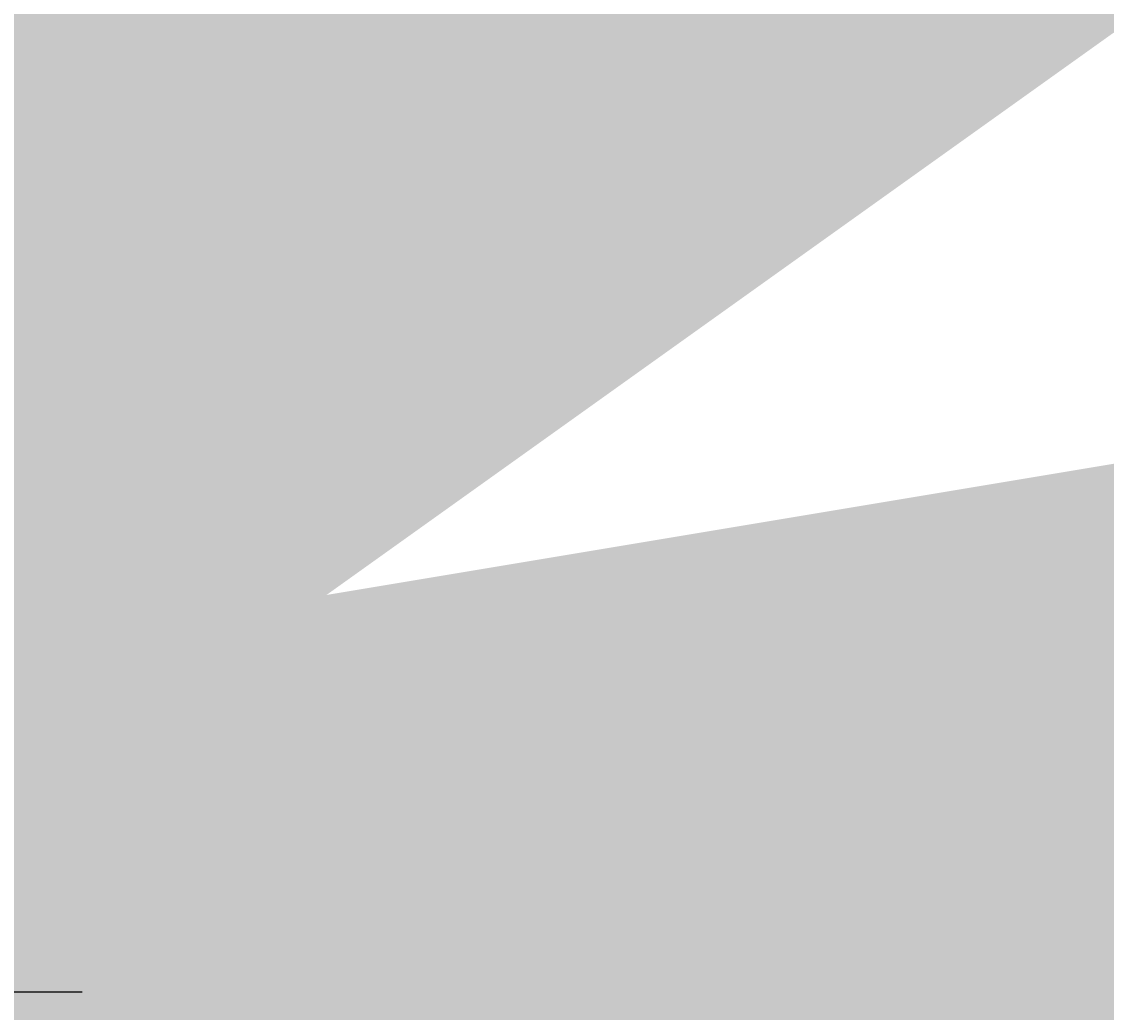
# Model space of a CAD drawing. Units: millimetres. Extents: x -22994 to 29398, y -19990 to 20176.
# Tile 126 of 135: x 296 to 480, y 173 to 341. Entities that reach past the tile are written whole.
import ezdxf

# ---------------------------------------------------------------- set-up
doc = ezdxf.new("R2010")
doc.units = ezdxf.units.MM
doc.header["$MEASUREMENT"] = 0
doc.layers.add('M-DIMS', color=2, linetype='Continuous', lineweight=18)
doc.styles.get("Standard").update_dxf_attribs({"font": 'arial.ttf'})
doc.dimstyles.get("Standard").update_dxf_attribs({"dimtxt": 0.18, "dimasz": 10000, "dimexe": 0.18, "dimexo": 0.0625, "dimgap": 0.09, "dimtad": 0, "dimtih": 1, "dimtoh": 1, "dimdec": 0, "dimzin": 0, "dimdsep": 46, "dimtxsty": 'Standard', "dimcen": 0.09, "dimadec": 0, "dimazin": 0, "dimtfac": 1, "dimtdec": 0, "dimtofl": 0, "dimtmove": 0, "dimatfit": 3, "dimfxl": 1, "dimtolj": 1, "dimtzin": 0, "dimlwd": 30, "dimarcsym": 0})

# ---------------------------------------------------------------- blocks, each defined once
blk = doc.blocks.new('*D2')
at = {"layer": 'Defpoints', "color": 0, "transparency": 16777216}
for p in [(6.68, 10.27), (290.85, 10.27), (290.85, -5.08)]:
    blk.add_point(p, dxfattribs=at)
at = {"layer": 'M-DIMS', "color": 0, "lineweight": -2, "transparency": 16777216}
for p, q in [((6.68, 10.21), (6.68, -5.26)), ((290.85, 10.21), (290.85, -5.26))]:
    blk.add_line(p, q, dxfattribs=at)
at = {"layer": 'M-DIMS', "color": 0, "lineweight": 30, "transparency": 16777216}
for p, q in [((-9993.32, -5.08), (-19993.32, -5.08)), ((10290.85, -5.08), (20290.85, -5.08))]:
    blk.add_line(p, q, dxfattribs=at)
at = {"layer": 'M-DIMS', "color": 0, "transparency": 16777216}
for points in [[(-9993.32, 1661.59), (-9993.32, -1671.75), (6.68, -5.08)], [(10290.85, 1661.59), (10290.85, -1671.75), (290.85, -5.08)]]:
    blk.add_solid(points, dxfattribs=at)
at = {"layer": 'M-DIMS', "color": 0, "transparency": 16777216, "insert": (148.76, -5.08), "char_height": 0.18, "attachment_point": 5}
blk.add_mtext('\\A1;284.2', dxfattribs=at)
blk = doc.blocks.new('*D3')
at = {"layer": 'Defpoints', "color": 0, "transparency": 16777216}
for p in [(110.26, 204.17), (110.26, 176.37), (95.83, 127.97)]:
    blk.add_point(p, dxfattribs=at)
at = {"layer": 'M-DIMS', "color": 0, "lineweight": 30, "transparency": 16777216}
for p, q in [((-9904.17, 204.17), (-19904.17, 204.17)), ((10110.26, 204.17), (20110.26, 204.17))]:
    blk.add_line(p, q, dxfattribs=at)
at = {"layer": 'M-DIMS', "color": 0, "lineweight": -2, "transparency": 16777216}
for p, q in [((95.83, 128.03), (95.83, 204.35)), ((110.26, 176.43), (110.26, 204.35))]:
    blk.add_line(p, q, dxfattribs=at)
at = {"layer": 'M-DIMS', "color": 0, "transparency": 16777216}
for points in [[(-9904.17, 1870.83), (-9904.17, -1462.5), (95.83, 204.17)], [(10110.26, 1870.83), (10110.26, -1462.5), (110.26, 204.17)]]:
    blk.add_solid(points, dxfattribs=at)
at = {"layer": 'M-DIMS', "color": 0, "transparency": 16777216, "insert": (103.05, 204.17), "char_height": 0.18, "attachment_point": 5}
blk.add_mtext('\\A1;14.432', dxfattribs=at)
blk = doc.blocks.new('*D4')
at = {"layer": 'Defpoints', "color": 0, "transparency": 16777216}
for p in [(116.26, 204.17), (110.26, 176.37), (116.26, 176.37)]:
    blk.add_point(p, dxfattribs=at)
at = {"layer": 'M-DIMS', "color": 0, "lineweight": 30, "transparency": 16777216}
for p, q in [((-9889.74, 204.17), (-19889.74, 204.17)), ((10116.26, 204.17), (20116.26, 204.17))]:
    blk.add_line(p, q, dxfattribs=at)
at = {"layer": 'M-DIMS', "color": 0, "lineweight": -2, "transparency": 16777216}
for p, q in [((110.26, 176.43), (110.26, 204.35)), ((116.26, 176.43), (116.26, 204.35))]:
    blk.add_line(p, q, dxfattribs=at)
at = {"layer": 'M-DIMS', "color": 0, "transparency": 16777216}
for points in [[(-9889.74, 1870.83), (-9889.74, -1462.5), (110.26, 204.17)], [(10116.26, 1870.83), (10116.26, -1462.5), (116.26, 204.17)]]:
    blk.add_solid(points, dxfattribs=at)
at = {"layer": 'M-DIMS', "color": 0, "transparency": 16777216, "insert": (113.26, 204.17), "char_height": 0.18, "attachment_point": 5}
blk.add_mtext('\\A1;6', dxfattribs=at)
blk = doc.blocks.new('*D5')
at = {"layer": 'Defpoints', "color": 0, "transparency": 16777216}
for p in [(181.26, 204.17), (116.26, 176.37), (181.26, 176.37)]:
    blk.add_point(p, dxfattribs=at)
at = {"layer": 'M-DIMS', "color": 0, "lineweight": 30, "transparency": 16777216}
for p, q in [((-9883.74, 204.17), (-19883.74, 204.17)), ((10181.26, 204.17), (20181.26, 204.17))]:
    blk.add_line(p, q, dxfattribs=at)
at = {"layer": 'M-DIMS', "color": 0, "lineweight": -2, "transparency": 16777216}
for p, q in [((116.26, 176.43), (116.26, 204.35)), ((181.26, 176.43), (181.26, 204.35))]:
    blk.add_line(p, q, dxfattribs=at)
at = {"layer": 'M-DIMS', "color": 0, "transparency": 16777216}
for points in [[(-9883.74, 1870.83), (-9883.74, -1462.5), (116.26, 204.17)], [(10181.26, 1870.83), (10181.26, -1462.5), (181.26, 204.17)]]:
    blk.add_solid(points, dxfattribs=at)
at = {"layer": 'M-DIMS', "color": 0, "transparency": 16777216, "insert": (148.76, 204.17), "char_height": 0.18, "attachment_point": 5}
blk.add_mtext('\\A1;65', dxfattribs=at)
blk = doc.blocks.new('*D6')
at = {"layer": 'Defpoints', "color": 0, "transparency": 16777216}
for p in [(187.26, 204.17), (181.26, 176.37), (187.26, 176.37)]:
    blk.add_point(p, dxfattribs=at)
at = {"layer": 'M-DIMS', "color": 0, "lineweight": 30, "transparency": 16777216}
for p, q in [((-9818.74, 204.17), (-19818.74, 204.17)), ((10187.26, 204.17), (20187.26, 204.17))]:
    blk.add_line(p, q, dxfattribs=at)
at = {"layer": 'M-DIMS', "color": 0, "lineweight": -2, "transparency": 16777216}
for p, q in [((181.26, 176.43), (181.26, 204.35)), ((187.26, 176.43), (187.26, 204.35))]:
    blk.add_line(p, q, dxfattribs=at)
at = {"layer": 'M-DIMS', "color": 0, "transparency": 16777216}
for points in [[(-9818.74, 1870.83), (-9818.74, -1462.5), (181.26, 204.17)], [(10187.26, 1870.83), (10187.26, -1462.5), (187.26, 204.17)]]:
    blk.add_solid(points, dxfattribs=at)
at = {"layer": 'M-DIMS', "color": 0, "transparency": 16777216, "insert": (184.26, 204.17), "char_height": 0.18, "attachment_point": 5}
blk.add_mtext('\\A1;6', dxfattribs=at)
blk = doc.blocks.new('*D7')
at = {"layer": 'Defpoints', "color": 0, "transparency": 16777216}
for p in [(201.7, 204.17), (187.26, 176.37), (201.7, 127.97)]:
    blk.add_point(p, dxfattribs=at)
at = {"layer": 'M-DIMS', "color": 0, "lineweight": 30, "transparency": 16777216}
for p, q in [((-9812.74, 204.17), (-19812.74, 204.17)), ((10201.7, 204.17), (20201.7, 204.17))]:
    blk.add_line(p, q, dxfattribs=at)
at = {"layer": 'M-DIMS', "color": 0, "lineweight": -2, "transparency": 16777216}
for p, q in [((187.26, 176.43), (187.26, 204.35)), ((201.7, 128.03), (201.7, 204.35))]:
    blk.add_line(p, q, dxfattribs=at)
at = {"layer": 'M-DIMS', "color": 0, "transparency": 16777216}
for points in [[(-9812.74, 1870.83), (-9812.74, -1462.5), (187.26, 204.17)], [(10201.7, 1870.83), (10201.7, -1462.5), (201.7, 204.17)]]:
    blk.add_solid(points, dxfattribs=at)
at = {"layer": 'M-DIMS', "color": 0, "transparency": 16777216, "insert": (194.48, 204.17), "char_height": 0.18, "attachment_point": 5}
blk.add_mtext('\\A1;14.432', dxfattribs=at)
blk = doc.blocks.new('*D8')
at = {"layer": 'Defpoints', "color": 0, "transparency": 16777216}
for p in [(227.65, 204.17), (227.65, 146.73), (201.7, 127.97)]:
    blk.add_point(p, dxfattribs=at)
at = {"layer": 'M-DIMS', "color": 0, "lineweight": 30, "transparency": 16777216}
for p, q in [((-9798.3, 204.17), (-19798.3, 204.17)), ((10227.65, 204.17), (20227.65, 204.17))]:
    blk.add_line(p, q, dxfattribs=at)
at = {"layer": 'M-DIMS', "color": 0, "lineweight": -2, "transparency": 16777216}
for p, q in [((201.7, 128.03), (201.7, 204.35)), ((227.65, 146.79), (227.65, 204.35))]:
    blk.add_line(p, q, dxfattribs=at)
at = {"layer": 'M-DIMS', "color": 0, "transparency": 16777216}
for points in [[(-9798.3, 1870.83), (-9798.3, -1462.5), (201.7, 204.17)], [(10227.65, 1870.83), (10227.65, -1462.5), (227.65, 204.17)]]:
    blk.add_solid(points, dxfattribs=at)
at = {"layer": 'M-DIMS', "color": 0, "transparency": 16777216, "insert": (214.67, 204.17), "char_height": 0.18, "attachment_point": 5}
blk.add_mtext('\\A1;25.95', dxfattribs=at)
blk = doc.blocks.new('*D9')
at = {"layer": 'Defpoints', "color": 0, "transparency": 16777216}
for p in [(187.26, 176.37), (306.2, 176.37), (290.85, 10.27)]:
    blk.add_point(p, dxfattribs=at)
at = {"layer": 'M-DIMS', "color": 0, "lineweight": 30, "transparency": 16777216}
for p, q in [((306.2, 10176.37), (306.2, 20176.37)), ((306.2, -9989.73), (306.2, -19989.73))]:
    blk.add_line(p, q, dxfattribs=at)
at = {"layer": 'M-DIMS', "color": 0, "lineweight": -2, "transparency": 16777216}
for p, q in [((187.33, 176.37), (306.38, 176.37)), ((290.91, 10.27), (306.38, 10.27))]:
    blk.add_line(p, q, dxfattribs=at)
at = {"layer": 'M-DIMS', "color": 0, "transparency": 16777216}
for points in [[(-1360.46, 10176.37), (1972.87, 10176.37), (306.2, 176.37)], [(-1360.46, -9989.73), (1972.87, -9989.73), (306.2, 10.27)]]:
    blk.add_solid(points, dxfattribs=at)
at = {"layer": 'M-DIMS', "color": 0, "transparency": 16777216, "insert": (306.2, 93.32), "char_height": 0.18, "attachment_point": 5}
blk.add_mtext('\\A1;166.1', dxfattribs=at)
blk = doc.blocks.new('*D10')
at = {"layer": 'Defpoints', "color": 0, "transparency": 16777216}
for p in [(125.65, 136.07), (133.35, 136.07), (133.35, -5.08)]:
    blk.add_point(p, dxfattribs=at)
at = {"layer": 'M-DIMS', "color": 0, "lineweight": -2, "transparency": 16777216}
for p, q in [((125.65, 136.01), (125.65, -5.26)), ((133.35, 136.01), (133.35, -5.26))]:
    blk.add_line(p, q, dxfattribs=at)
at = {"layer": 'M-DIMS', "color": 0, "lineweight": 30, "transparency": 16777216}
for p, q in [((-9874.35, -5.08), (-19874.35, -5.08)), ((10133.35, -5.08), (20133.35, -5.08))]:
    blk.add_line(p, q, dxfattribs=at)
at = {"layer": 'M-DIMS', "color": 0, "transparency": 16777216}
for points in [[(-9874.35, 1661.59), (-9874.35, -1671.75), (125.65, -5.08)], [(10133.35, 1661.59), (10133.35, -1671.75), (133.35, -5.08)]]:
    blk.add_solid(points, dxfattribs=at)
at = {"layer": 'M-DIMS', "color": 0, "transparency": 16777216, "insert": (129.5, -5.08), "char_height": 0.18, "attachment_point": 5}
blk.add_mtext('\\A1;7.696', dxfattribs=at)
blk = doc.blocks.new('*D11')
at = {"layer": 'Defpoints', "color": 0, "transparency": 16777216}
for p in [(133.35, 136.07), (135.65, 136.07), (135.65, -5.08)]:
    blk.add_point(p, dxfattribs=at)
at = {"layer": 'M-DIMS', "color": 0, "lineweight": -2, "transparency": 16777216}
for p, q in [((133.35, 136.01), (133.35, -5.26)), ((135.65, 136.01), (135.65, -5.26))]:
    blk.add_line(p, q, dxfattribs=at)
at = {"layer": 'M-DIMS', "color": 0, "lineweight": 30, "transparency": 16777216}
for p, q in [((-9866.65, -5.08), (-19866.65, -5.08)), ((10135.65, -5.08), (20135.65, -5.08))]:
    blk.add_line(p, q, dxfattribs=at)
at = {"layer": 'M-DIMS', "color": 0, "transparency": 16777216}
for points in [[(-9866.65, 1661.59), (-9866.65, -1671.75), (133.35, -5.08)], [(10135.65, 1661.59), (10135.65, -1671.75), (135.65, -5.08)]]:
    blk.add_solid(points, dxfattribs=at)
at = {"layer": 'M-DIMS', "color": 0, "transparency": 16777216, "insert": (134.5, -5.08), "char_height": 0.18, "attachment_point": 5}
blk.add_mtext('\\A1;2.304', dxfattribs=at)
blk = doc.blocks.new('*D12')
at = {"layer": 'Defpoints', "color": 0, "transparency": 16777216}
for p in [(135.65, 136.07), (145.65, 136.07), (145.65, -5.08)]:
    blk.add_point(p, dxfattribs=at)
at = {"layer": 'M-DIMS', "color": 0, "lineweight": -2, "transparency": 16777216}
for p, q in [((135.65, 136.01), (135.65, -5.26)), ((145.65, 136.01), (145.65, -5.26))]:
    blk.add_line(p, q, dxfattribs=at)
at = {"layer": 'M-DIMS', "color": 0, "lineweight": 30, "transparency": 16777216}
for p, q in [((-9864.35, -5.08), (-19864.35, -5.08)), ((10145.65, -5.08), (20145.65, -5.08))]:
    blk.add_line(p, q, dxfattribs=at)
at = {"layer": 'M-DIMS', "color": 0, "transparency": 16777216}
for points in [[(-9864.35, 1661.59), (-9864.35, -1671.75), (135.65, -5.08)], [(10145.65, 1661.59), (10145.65, -1671.75), (145.65, -5.08)]]:
    blk.add_solid(points, dxfattribs=at)
at = {"layer": 'M-DIMS', "color": 0, "transparency": 16777216, "insert": (140.65, -5.08), "char_height": 0.18, "attachment_point": 5}
blk.add_mtext('\\A1;10', dxfattribs=at)
blk = doc.blocks.new('*D13')
at = {"layer": 'Defpoints', "color": 0, "transparency": 16777216}
for p in [(145.65, 136.07), (155.65, 136.07), (155.65, -5.08)]:
    blk.add_point(p, dxfattribs=at)
at = {"layer": 'M-DIMS', "color": 0, "lineweight": -2, "transparency": 16777216}
for p, q in [((145.65, 136.01), (145.65, -5.26)), ((155.65, 136.01), (155.65, -5.26))]:
    blk.add_line(p, q, dxfattribs=at)
at = {"layer": 'M-DIMS', "color": 0, "lineweight": 30, "transparency": 16777216}
for p, q in [((-9854.35, -5.08), (-19854.35, -5.08)), ((10155.65, -5.08), (20155.65, -5.08))]:
    blk.add_line(p, q, dxfattribs=at)
at = {"layer": 'M-DIMS', "color": 0, "transparency": 16777216}
for points in [[(-9854.35, 1661.59), (-9854.35, -1671.75), (145.65, -5.08)], [(10155.65, 1661.59), (10155.65, -1671.75), (155.65, -5.08)]]:
    blk.add_solid(points, dxfattribs=at)
at = {"layer": 'M-DIMS', "color": 0, "transparency": 16777216, "insert": (150.65, -5.08), "char_height": 0.18, "attachment_point": 5}
blk.add_mtext('\\A1;10', dxfattribs=at)
blk = doc.blocks.new('*D14')
at = {"layer": 'Defpoints', "color": 0, "transparency": 16777216}
for p in [(155.65, 136.07), (165.65, 136.07), (165.65, -5.08)]:
    blk.add_point(p, dxfattribs=at)
at = {"layer": 'M-DIMS', "color": 0, "lineweight": -2, "transparency": 16777216}
for p, q in [((155.65, 136.01), (155.65, -5.26)), ((165.65, 136.01), (165.65, -5.26))]:
    blk.add_line(p, q, dxfattribs=at)
at = {"layer": 'M-DIMS', "color": 0, "lineweight": 30, "transparency": 16777216}
for p, q in [((-9844.35, -5.08), (-19844.35, -5.08)), ((10165.65, -5.08), (20165.65, -5.08))]:
    blk.add_line(p, q, dxfattribs=at)
at = {"layer": 'M-DIMS', "color": 0, "transparency": 16777216}
for points in [[(-9844.35, 1661.59), (-9844.35, -1671.75), (155.65, -5.08)], [(10165.65, 1661.59), (10165.65, -1671.75), (165.65, -5.08)]]:
    blk.add_solid(points, dxfattribs=at)
at = {"layer": 'M-DIMS', "color": 0, "transparency": 16777216, "insert": (160.65, -5.08), "char_height": 0.18, "attachment_point": 5}
blk.add_mtext('\\A1;10', dxfattribs=at)
blk = doc.blocks.new('*D15')
at = {"layer": 'Defpoints', "color": 0, "transparency": 16777216}
for p in [(173.35, 154.79), (173.35, 136.07), (306.2, 136.07)]:
    blk.add_point(p, dxfattribs=at)
at = {"layer": 'M-DIMS', "color": 0, "lineweight": 30, "transparency": 16777216}
for p, q in [((306.2, 10154.79), (306.2, 20154.79)), ((306.2, -9863.93), (306.2, -19863.93))]:
    blk.add_line(p, q, dxfattribs=at)
at = {"layer": 'M-DIMS', "color": 0, "lineweight": -2, "transparency": 16777216}
for p, q in [((173.41, 154.79), (306.38, 154.79)), ((173.41, 136.07), (306.38, 136.07))]:
    blk.add_line(p, q, dxfattribs=at)
at = {"layer": 'M-DIMS', "color": 0, "transparency": 16777216}
for points in [[(-1360.46, 10154.79), (1972.87, 10154.79), (306.2, 154.79)], [(-1360.46, -9863.93), (1972.87, -9863.93), (306.2, 136.07)]]:
    blk.add_solid(points, dxfattribs=at)
at = {"layer": 'M-DIMS', "color": 0, "transparency": 16777216, "insert": (306.2, 145.43), "char_height": 0.18, "attachment_point": 5}
blk.add_mtext('\\A1;18.717', dxfattribs=at)
blk = doc.blocks.new('*D16')
at = {"layer": 'Defpoints', "color": 0, "transparency": 16777216}
for p in [(120.17, 204.17), (110.47, 48.03), (120.17, 48.03)]:
    blk.add_point(p, dxfattribs=at)
at = {"layer": 'M-DIMS', "color": 0, "lineweight": 30, "transparency": 16777216}
for p, q in [((-9889.53, 204.17), (-19889.53, 204.17)), ((10120.17, 204.17), (20120.17, 204.17))]:
    blk.add_line(p, q, dxfattribs=at)
at = {"layer": 'M-DIMS', "color": 0, "lineweight": -2, "transparency": 16777216}
for p, q in [((110.47, 48.1), (110.47, 204.35)), ((120.17, 48.1), (120.17, 204.35))]:
    blk.add_line(p, q, dxfattribs=at)
at = {"layer": 'M-DIMS', "color": 0, "transparency": 16777216}
for points in [[(-9889.53, 1870.83), (-9889.53, -1462.5), (110.47, 204.17)], [(10120.17, 1870.83), (10120.17, -1462.5), (120.17, 204.17)]]:
    blk.add_solid(points, dxfattribs=at)
at = {"layer": 'M-DIMS', "color": 0, "transparency": 16777216, "insert": (115.32, 204.17), "char_height": 0.18, "attachment_point": 5}
blk.add_mtext('\\A1;9.704', dxfattribs=at)
blk = doc.blocks.new('*D17')
at = {"layer": 'Defpoints', "color": 0, "transparency": 16777216}
for p in [(126.17, 204.17), (120.17, 48.03), (126.17, 48.03)]:
    blk.add_point(p, dxfattribs=at)
at = {"layer": 'M-DIMS', "color": 0, "lineweight": 30, "transparency": 16777216}
for p, q in [((-9879.83, 204.17), (-19879.83, 204.17)), ((10126.17, 204.17), (20126.17, 204.17))]:
    blk.add_line(p, q, dxfattribs=at)
at = {"layer": 'M-DIMS', "color": 0, "lineweight": -2, "transparency": 16777216}
for p, q in [((120.17, 48.1), (120.17, 204.35)), ((126.17, 48.1), (126.17, 204.35))]:
    blk.add_line(p, q, dxfattribs=at)
at = {"layer": 'M-DIMS', "color": 0, "transparency": 16777216}
for points in [[(-9879.83, 1870.83), (-9879.83, -1462.5), (120.17, 204.17)], [(10126.17, 1870.83), (10126.17, -1462.5), (126.17, 204.17)]]:
    blk.add_solid(points, dxfattribs=at)
at = {"layer": 'M-DIMS', "color": 0, "transparency": 16777216, "insert": (123.17, 204.17), "char_height": 0.18, "attachment_point": 5}
blk.add_mtext('\\A1;6', dxfattribs=at)
blk = doc.blocks.new('*D18')
at = {"layer": 'Defpoints', "color": 0, "transparency": 16777216}
for p in [(132.17, 204.17), (126.17, 48.03), (132.17, 48.03)]:
    blk.add_point(p, dxfattribs=at)
at = {"layer": 'M-DIMS', "color": 0, "lineweight": 30, "transparency": 16777216}
for p, q in [((-9873.83, 204.17), (-19873.83, 204.17)), ((10132.17, 204.17), (20132.17, 204.17))]:
    blk.add_line(p, q, dxfattribs=at)
at = {"layer": 'M-DIMS', "color": 0, "lineweight": -2, "transparency": 16777216}
for p, q in [((126.17, 48.1), (126.17, 204.35)), ((132.17, 48.1), (132.17, 204.35))]:
    blk.add_line(p, q, dxfattribs=at)
at = {"layer": 'M-DIMS', "color": 0, "transparency": 16777216}
for points in [[(-9873.83, 1870.83), (-9873.83, -1462.5), (126.17, 204.17)], [(10132.17, 1870.83), (10132.17, -1462.5), (132.17, 204.17)]]:
    blk.add_solid(points, dxfattribs=at)
at = {"layer": 'M-DIMS', "color": 0, "transparency": 16777216, "insert": (129.17, 204.17), "char_height": 0.18, "attachment_point": 5}
blk.add_mtext('\\A1;6', dxfattribs=at)
blk = doc.blocks.new('*D19')
at = {"layer": 'Defpoints', "color": 0, "transparency": 16777216}
for p in [(138.17, 204.17), (132.17, 48.03), (138.17, 48.03)]:
    blk.add_point(p, dxfattribs=at)
at = {"layer": 'M-DIMS', "color": 0, "lineweight": 30, "transparency": 16777216}
for p, q in [((-9867.83, 204.17), (-19867.83, 204.17)), ((10138.17, 204.17), (20138.17, 204.17))]:
    blk.add_line(p, q, dxfattribs=at)
at = {"layer": 'M-DIMS', "color": 0, "lineweight": -2, "transparency": 16777216}
for p, q in [((132.17, 48.1), (132.17, 204.35)), ((138.17, 48.1), (138.17, 204.35))]:
    blk.add_line(p, q, dxfattribs=at)
at = {"layer": 'M-DIMS', "color": 0, "transparency": 16777216}
for points in [[(-9867.83, 1870.83), (-9867.83, -1462.5), (132.17, 204.17)], [(10138.17, 1870.83), (10138.17, -1462.5), (138.17, 204.17)]]:
    blk.add_solid(points, dxfattribs=at)
at = {"layer": 'M-DIMS', "color": 0, "transparency": 16777216, "insert": (135.17, 204.17), "char_height": 0.18, "attachment_point": 5}
blk.add_mtext('\\A1;6', dxfattribs=at)
blk = doc.blocks.new('*D20')
at = {"layer": 'Defpoints', "color": 0, "transparency": 16777216}
for p in [(144.17, 204.17), (138.17, 48.03), (144.17, 48.03)]:
    blk.add_point(p, dxfattribs=at)
at = {"layer": 'M-DIMS', "color": 0, "lineweight": 30, "transparency": 16777216}
for p, q in [((-9861.83, 204.17), (-19861.83, 204.17)), ((10144.17, 204.17), (20144.17, 204.17))]:
    blk.add_line(p, q, dxfattribs=at)
at = {"layer": 'M-DIMS', "color": 0, "lineweight": -2, "transparency": 16777216}
for p, q in [((138.17, 48.1), (138.17, 204.35)), ((144.17, 48.1), (144.17, 204.35))]:
    blk.add_line(p, q, dxfattribs=at)
at = {"layer": 'M-DIMS', "color": 0, "transparency": 16777216}
for points in [[(-9861.83, 1870.83), (-9861.83, -1462.5), (138.17, 204.17)], [(10144.17, 1870.83), (10144.17, -1462.5), (144.17, 204.17)]]:
    blk.add_solid(points, dxfattribs=at)
at = {"layer": 'M-DIMS', "color": 0, "transparency": 16777216, "insert": (141.17, 204.17), "char_height": 0.18, "attachment_point": 5}
blk.add_mtext('\\A1;6', dxfattribs=at)
blk = doc.blocks.new('*D21')
at = {"layer": 'Defpoints', "color": 0, "transparency": 16777216}
for p in [(149.12, 204.17), (144.17, 48.03), (149.12, 48.03)]:
    blk.add_point(p, dxfattribs=at)
at = {"layer": 'M-DIMS', "color": 0, "lineweight": 30, "transparency": 16777216}
for p, q in [((-9855.83, 204.17), (-19855.83, 204.17)), ((10149.12, 204.17), (20149.12, 204.17))]:
    blk.add_line(p, q, dxfattribs=at)
at = {"layer": 'M-DIMS', "color": 0, "lineweight": -2, "transparency": 16777216}
for p, q in [((144.17, 48.1), (144.17, 204.35)), ((149.12, 48.1), (149.12, 204.35))]:
    blk.add_line(p, q, dxfattribs=at)
at = {"layer": 'M-DIMS', "color": 0, "transparency": 16777216}
for points in [[(-9855.83, 1870.83), (-9855.83, -1462.5), (144.17, 204.17)], [(10149.12, 1870.83), (10149.12, -1462.5), (149.12, 204.17)]]:
    blk.add_solid(points, dxfattribs=at)
at = {"layer": 'M-DIMS', "color": 0, "transparency": 16777216, "insert": (146.64, 204.17), "char_height": 0.18, "attachment_point": 5}
blk.add_mtext('\\A1;4.945', dxfattribs=at)
blk = doc.blocks.new('*D22')
at = {"layer": 'Defpoints', "color": 0, "transparency": 16777216}
for p in [(149.12, 30.99), (155.12, 30.99), (155.12, -5.08)]:
    blk.add_point(p, dxfattribs=at)
at = {"layer": 'M-DIMS', "color": 0, "lineweight": -2, "transparency": 16777216}
for p, q in [((149.12, 30.93), (149.12, -5.26)), ((155.12, 30.93), (155.12, -5.26))]:
    blk.add_line(p, q, dxfattribs=at)
at = {"layer": 'M-DIMS', "color": 0, "lineweight": 30, "transparency": 16777216}
for p, q in [((-9850.88, -5.08), (-19850.88, -5.08)), ((10155.12, -5.08), (20155.12, -5.08))]:
    blk.add_line(p, q, dxfattribs=at)
at = {"layer": 'M-DIMS', "color": 0, "transparency": 16777216}
for points in [[(-9850.88, 1661.59), (-9850.88, -1671.75), (149.12, -5.08)], [(10155.12, 1661.59), (10155.12, -1671.75), (155.12, -5.08)]]:
    blk.add_solid(points, dxfattribs=at)
at = {"layer": 'M-DIMS', "color": 0, "transparency": 16777216, "insert": (152.12, -5.08), "char_height": 0.18, "attachment_point": 5}
blk.add_mtext('\\A1;6', dxfattribs=at)
blk = doc.blocks.new('*D23')
at = {"layer": 'Defpoints', "color": 0, "transparency": 16777216}
for p in [(155.12, 30.99), (161.12, 30.99), (161.12, -5.08)]:
    blk.add_point(p, dxfattribs=at)
at = {"layer": 'M-DIMS', "color": 0, "lineweight": -2, "transparency": 16777216}
for p, q in [((155.12, 30.93), (155.12, -5.26)), ((161.12, 30.93), (161.12, -5.26))]:
    blk.add_line(p, q, dxfattribs=at)
at = {"layer": 'M-DIMS', "color": 0, "lineweight": 30, "transparency": 16777216}
for p, q in [((-9844.88, -5.08), (-19844.88, -5.08)), ((10161.12, -5.08), (20161.12, -5.08))]:
    blk.add_line(p, q, dxfattribs=at)
at = {"layer": 'M-DIMS', "color": 0, "transparency": 16777216}
for points in [[(-9844.88, 1661.59), (-9844.88, -1671.75), (155.12, -5.08)], [(10161.12, 1661.59), (10161.12, -1671.75), (161.12, -5.08)]]:
    blk.add_solid(points, dxfattribs=at)
at = {"layer": 'M-DIMS', "color": 0, "transparency": 16777216, "insert": (158.12, -5.08), "char_height": 0.18, "attachment_point": 5}
blk.add_mtext('\\A1;6', dxfattribs=at)
blk = doc.blocks.new('*D24')
at = {"layer": 'Defpoints', "color": 0, "transparency": 16777216}
for p in [(161.12, 30.99), (166.44, 30.99), (166.44, -5.08)]:
    blk.add_point(p, dxfattribs=at)
at = {"layer": 'M-DIMS', "color": 0, "lineweight": -2, "transparency": 16777216}
for p, q in [((161.12, 30.93), (161.12, -5.26)), ((166.44, 30.93), (166.44, -5.26))]:
    blk.add_line(p, q, dxfattribs=at)
at = {"layer": 'M-DIMS', "color": 0, "lineweight": 30, "transparency": 16777216}
for p, q in [((-9838.88, -5.08), (-19838.88, -5.08)), ((10166.44, -5.08), (20166.44, -5.08))]:
    blk.add_line(p, q, dxfattribs=at)
at = {"layer": 'M-DIMS', "color": 0, "transparency": 16777216}
for points in [[(-9838.88, 1661.59), (-9838.88, -1671.75), (161.12, -5.08)], [(10166.44, 1661.59), (10166.44, -1671.75), (166.44, -5.08)]]:
    blk.add_solid(points, dxfattribs=at)
at = {"layer": 'M-DIMS', "color": 0, "transparency": 16777216, "insert": (163.78, -5.08), "char_height": 0.18, "attachment_point": 5}
blk.add_mtext('\\A1;5.323', dxfattribs=at)
blk = doc.blocks.new('*D25')
at = {"layer": 'Defpoints', "color": 0, "transparency": 16777216}
for p in [(166.44, 30.99), (172.44, 30.99), (172.44, -5.08)]:
    blk.add_point(p, dxfattribs=at)
at = {"layer": 'M-DIMS', "color": 0, "lineweight": -2, "transparency": 16777216}
for p, q in [((166.44, 30.93), (166.44, -5.26)), ((172.44, 30.93), (172.44, -5.26))]:
    blk.add_line(p, q, dxfattribs=at)
at = {"layer": 'M-DIMS', "color": 0, "lineweight": 30, "transparency": 16777216}
for p, q in [((-9833.56, -5.08), (-19833.56, -5.08)), ((10172.44, -5.08), (20172.44, -5.08))]:
    blk.add_line(p, q, dxfattribs=at)
at = {"layer": 'M-DIMS', "color": 0, "transparency": 16777216}
for points in [[(-9833.56, 1661.59), (-9833.56, -1671.75), (166.44, -5.08)], [(10172.44, 1661.59), (10172.44, -1671.75), (172.44, -5.08)]]:
    blk.add_solid(points, dxfattribs=at)
at = {"layer": 'M-DIMS', "color": 0, "transparency": 16777216, "insert": (169.44, -5.08), "char_height": 0.18, "attachment_point": 5}
blk.add_mtext('\\A1;6', dxfattribs=at)
blk = doc.blocks.new('*D26')
at = {"layer": 'Defpoints', "color": 0, "transparency": 16777216}
for p in [(172.44, 30.99), (178.44, 30.99), (178.44, -5.08)]:
    blk.add_point(p, dxfattribs=at)
at = {"layer": 'M-DIMS', "color": 0, "lineweight": -2, "transparency": 16777216}
for p, q in [((172.44, 30.93), (172.44, -5.26)), ((178.44, 30.93), (178.44, -5.26))]:
    blk.add_line(p, q, dxfattribs=at)
at = {"layer": 'M-DIMS', "color": 0, "lineweight": 30, "transparency": 16777216}
for p, q in [((-9827.56, -5.08), (-19827.56, -5.08)), ((10178.44, -5.08), (20178.44, -5.08))]:
    blk.add_line(p, q, dxfattribs=at)
at = {"layer": 'M-DIMS', "color": 0, "transparency": 16777216}
for points in [[(-9827.56, 1661.59), (-9827.56, -1671.75), (172.44, -5.08)], [(10178.44, 1661.59), (10178.44, -1671.75), (178.44, -5.08)]]:
    blk.add_solid(points, dxfattribs=at)
at = {"layer": 'M-DIMS', "color": 0, "transparency": 16777216, "insert": (175.44, -5.08), "char_height": 0.18, "attachment_point": 5}
blk.add_mtext('\\A1;6', dxfattribs=at)
blk = doc.blocks.new('*D27')
at = {"layer": 'Defpoints', "color": 0, "transparency": 16777216}
for p in [(178.44, 30.99), (188.12, 30.99), (188.12, -5.08)]:
    blk.add_point(p, dxfattribs=at)
at = {"layer": 'M-DIMS', "color": 0, "lineweight": -2, "transparency": 16777216}
for p, q in [((178.44, 30.93), (178.44, -5.26)), ((188.12, 30.93), (188.12, -5.26))]:
    blk.add_line(p, q, dxfattribs=at)
at = {"layer": 'M-DIMS', "color": 0, "lineweight": 30, "transparency": 16777216}
for p, q in [((-9821.56, -5.08), (-19821.56, -5.08)), ((10188.12, -5.08), (20188.12, -5.08))]:
    blk.add_line(p, q, dxfattribs=at)
at = {"layer": 'M-DIMS', "color": 0, "transparency": 16777216}
for points in [[(-9821.56, 1661.59), (-9821.56, -1671.75), (178.44, -5.08)], [(10188.12, 1661.59), (10188.12, -1671.75), (188.12, -5.08)]]:
    blk.add_solid(points, dxfattribs=at)
at = {"layer": 'M-DIMS', "color": 0, "transparency": 16777216, "insert": (183.28, -5.08), "char_height": 0.18, "attachment_point": 5}
blk.add_mtext('\\A1;9.679', dxfattribs=at)
blk = doc.blocks.new('*D28')
at = {"layer": 'Defpoints', "color": 0, "transparency": 16777216}
for p in [(188.12, 48.03), (306.2, 48.03), (188.12, 30.99)]:
    blk.add_point(p, dxfattribs=at)
at = {"layer": 'M-DIMS', "color": 0, "lineweight": 30, "transparency": 16777216}
for p, q in [((306.2, 10048.03), (306.2, 20048.03)), ((306.2, -9969.01), (306.2, -19969.01))]:
    blk.add_line(p, q, dxfattribs=at)
at = {"layer": 'M-DIMS', "color": 0, "lineweight": -2, "transparency": 16777216}
for p, q in [((188.18, 48.03), (306.38, 48.03)), ((188.18, 30.99), (306.38, 30.99))]:
    blk.add_line(p, q, dxfattribs=at)
at = {"layer": 'M-DIMS', "color": 0, "transparency": 16777216}
for points in [[(-1360.46, 10048.03), (1972.87, 10048.03), (306.2, 48.03)], [(-1360.46, -9969.01), (1972.87, -9969.01), (306.2, 30.99)]]:
    blk.add_solid(points, dxfattribs=at)
at = {"layer": 'M-DIMS', "color": 0, "transparency": 16777216, "insert": (306.2, 39.51), "char_height": 0.18, "attachment_point": 5}
blk.add_mtext('\\A1;17.045', dxfattribs=at)
blk = doc.blocks.new('*D29')
at = {"layer": 'Defpoints', "color": 0, "transparency": 16777216}
for p in [(36.8, 80.04), (64.03, 80.04)]:
    blk.add_point(p, dxfattribs=at)
at = {"layer": 'M-DIMS', "color": 0, "lineweight": -2, "transparency": 16777216}
for p, q in [((50.33, 80.04), (50.51, 80.04)), ((50.42, 79.96), (50.42, 80.14))]:
    blk.add_line(p, q, dxfattribs=at)
at = {"layer": 'M-DIMS', "color": 0, "lineweight": 30, "transparency": 16777216}
blk.add_line((20064.03, 80.03), (10064.03, 80.04), dxfattribs=at)
at = {"layer": 'M-DIMS', "color": 0, "transparency": 16777216}
blk.add_solid([(10064.03, 1746.7), (10064.03, -1586.63), (64.03, 80.04)], dxfattribs=at)
at = {"layer": 'M-DIMS', "color": 0, "transparency": 16777216, "insert": (20064.52, 80.03), "char_height": 0.18, "attachment_point": 5}
blk.add_mtext('\\A1;∅27.23', dxfattribs=at)
blk = doc.blocks.new('*D30')
at = {"layer": 'Defpoints', "color": 0, "transparency": 16777216}
for p in [(216.31, 146.73), (238.98, 146.73)]:
    blk.add_point(p, dxfattribs=at)
at = {"layer": 'M-DIMS', "color": 0, "lineweight": 30, "transparency": 16777216}
blk.add_line((20238.98, 147.5), (10238.98, 147.11), dxfattribs=at)
at = {"layer": 'M-DIMS', "color": 0, "lineweight": -2, "transparency": 16777216}
for p, q in [((227.56, 146.73), (227.74, 146.73)), ((227.65, 146.64), (227.65, 146.82))]:
    blk.add_line(p, q, dxfattribs=at)
at = {"layer": 'M-DIMS', "color": 0, "transparency": 16777216}
blk.add_solid([(10238.92, 1813.78), (10239.05, -1519.55), (238.98, 146.73)], dxfattribs=at)
at = {"layer": 'M-DIMS', "color": 0, "transparency": 16777216, "insert": (20239.54, 147.5), "char_height": 0.18, "attachment_point": 5}
blk.add_mtext('\\A1;∅22.667', dxfattribs=at)
blk = doc.blocks.new('*D31')
at = {"layer": 'Defpoints', "color": 0, "transparency": 16777216}
for p in [(223.16, 146.73), (232.13, 146.73)]:
    blk.add_point(p, dxfattribs=at)
at = {"layer": 'M-DIMS', "color": 0, "lineweight": 30, "transparency": 16777216}
blk.add_line((20232.13, 148.67), (10232.13, 147.7), dxfattribs=at)
at = {"layer": 'M-DIMS', "color": 0, "lineweight": -2, "transparency": 16777216}
for p, q in [((227.56, 146.73), (227.74, 146.73)), ((227.65, 146.64), (227.65, 146.82))]:
    blk.add_line(p, q, dxfattribs=at)
at = {"layer": 'M-DIMS', "color": 0, "transparency": 16777216}
blk.add_solid([(10231.97, 1814.36), (10232.29, -1518.97), (232.13, 146.73)], dxfattribs=at)
at = {"layer": 'M-DIMS', "color": 0, "transparency": 16777216, "insert": (20232.62, 148.67), "char_height": 0.18, "attachment_point": 5}
blk.add_mtext('\\A1;∅8.969', dxfattribs=at)
blk = doc.blocks.new('*D34')
at = {"layer": 'Defpoints', "color": 0, "transparency": 16777216}
for p in [(178.58, 122.9), (176.81, 121.13)]:
    blk.add_point(p, dxfattribs=at)
at = {"layer": 'M-DIMS', "color": 0, "lineweight": 30, "transparency": 16777216}
for p, q in [((14322.44, 14263.31), (7250.51, 7193.1)), ((24322.44, 14263.31), (14322.44, 14263.31))]:
    blk.add_line(p, q, dxfattribs=at)
at = {"layer": 'M-DIMS', "color": 0, "lineweight": -2, "transparency": 16777216}
for p, q in [((176.72, 121.13), (176.9, 121.13)), ((176.81, 121.04), (176.81, 121.22))]:
    blk.add_line(p, q, dxfattribs=at)
at = {"layer": 'M-DIMS', "color": 0, "transparency": 16777216}
blk.add_solid([(6072.14, 8371.76), (8428.88, 6014.45), (178.58, 122.9)], dxfattribs=at)
at = {"layer": 'M-DIMS', "color": 0, "transparency": 16777216, "insert": (24322.97, 14263.31), "char_height": 0.18, "attachment_point": 5}
blk.add_mtext('\\A1;6X R2.5', dxfattribs=at)
blk = doc.blocks.new('*D36')
at = {"layer": 'Defpoints', "color": 0, "transparency": 16777216}
for p in [(46.39, 31.3), (46.39, 26.59)]:
    blk.add_point(p, dxfattribs=at)
at = {"layer": 'M-DIMS', "color": 0, "lineweight": 30, "transparency": 16777216}
for p, q in [((57.15, 20031.3), (51.77, 10031.3)), ((10057.15, 20031.3), (57.15, 20031.3))]:
    blk.add_line(p, q, dxfattribs=at)
at = {"layer": 'M-DIMS', "color": 0, "lineweight": -2, "transparency": 16777216}
for p, q in [((46.3, 28.95), (46.48, 28.95)), ((46.39, 28.86), (46.39, 29.04))]:
    blk.add_line(p, q, dxfattribs=at)
at = {"layer": 'M-DIMS', "color": 0, "transparency": 16777216}
blk.add_solid([(-1614.9, 10032.2), (1718.44, 10030.41), (46.39, 31.3)], dxfattribs=at)
at = {"layer": 'M-DIMS', "color": 0, "transparency": 16777216, "insert": (10057.55, 20031.3), "char_height": 0.18, "attachment_point": 5}
blk.add_mtext('\\A1;∅4.71', dxfattribs=at)
blk = doc.blocks.new('*D37')
at = {"layer": 'Defpoints', "color": 0, "transparency": 16777216}
for p in [(54.83, 118.61), (59.49, 118.61)]:
    blk.add_point(p, dxfattribs=at)
at = {"layer": 'M-DIMS', "color": 0, "lineweight": -2, "transparency": 16777216}
for p, q in [((57.07, 118.61), (57.25, 118.61)), ((57.16, 118.52), (57.16, 118.7))]:
    blk.add_line(p, q, dxfattribs=at)
at = {"layer": 'M-DIMS', "color": 0, "lineweight": 30, "transparency": 16777216}
blk.add_line((20059.49, 116.25), (10059.49, 117.43), dxfattribs=at)
at = {"layer": 'M-DIMS', "color": 0, "transparency": 16777216}
blk.add_solid([(10059.69, 1784.1), (10059.3, -1549.23), (59.49, 118.61)], dxfattribs=at)
at = {"layer": 'M-DIMS', "color": 0, "transparency": 16777216, "insert": (20059.99, 116.25), "char_height": 0.18, "attachment_point": 5}
blk.add_mtext('\\A1;∅4.659', dxfattribs=at)

msp = doc.modelspace()

# ---------------------------------------------------------------- dimensions: what is measured, and where the dimension line sits
at = {"layer": 'M-DIMS'}
for base, p1, p2, override, picture, middle in [((306.202, 176.3662), (290.852, 10.2713), (187.2647, 176.3662), {"dimdec": 1, "dimlfac": 1, "dimrnd": 0, "dimzin": 0, "dimdsep": 46, "dimlunit": 2}, '*D9', (306.202, 93.3187)), ((306.202, 136.0713), (173.3459, 154.788), (173.3459, 136.0713), {"dimdec": 3, "dimlfac": 1, "dimrnd": 0, "dimzin": 0, "dimdsep": 46, "dimlunit": 2}, '*D15', (306.202, 145.4297)), ((306.202, 48.0349), (188.1175, 30.9895), (188.1175, 48.0349), {"dimdec": 3, "dimlfac": 1, "dimrnd": 0, "dimzin": 0, "dimdsep": 46, "dimlunit": 2}, '*D28', (306.202, 39.5122))]:
    dim = msp.add_linear_dim(base=base, p1=p1, p2=p2, angle=90, dimstyle='Standard', override=override, dxfattribs=at)
    dim.commit()
    dim.dimension.update_dxf_attribs({"geometry": picture, "text_midpoint": middle})
for p1, p2, override, picture, middle in [((46.3875, 26.5934), (46.39, 31.3035), {"dimdec": 2, "dimlfac": 1, "dimrnd": 0, "dimzin": 0, "dimdsep": 46, "dimlunit": 2}, '*D36', (10057.5542, 20031.3006)), ((223.1641, 146.7291), (232.1328, 146.73), {"dimdec": 3, "dimlfac": 1, "dimrnd": 0, "dimzin": 0, "dimdsep": 46, "dimlunit": 2}, '*D31', (20232.1327, 148.6656)), ((216.3148, 146.7291), (238.9821, 146.73), {"dimdec": 3, "dimlfac": 1, "dimrnd": 0, "dimzin": 0, "dimdsep": 46, "dimlunit": 2}, '*D30', (20238.9821, 147.4959))]:
    dim = msp.add_diameter_dim_2p(p1=p1, p2=p2, dimstyle='Standard', override=override, dxfattribs=at)
    dim.commit()
    dim.dimension.update_dxf_attribs({"geometry": picture, "text_midpoint": middle, "dimtype": 163})
dim = msp.add_radius_dim(center=(176.8123, 121.1277), mpoint=(178.5802, 122.8952), text='6X <>', dimstyle='Standard', override={"dimdec": 1, "dimlfac": 1, "dimrnd": 0, "dimzin": 0, "dimdsep": 46, "dimlunit": 2}, dxfattribs=at)
dim.commit()
dim.dimension.update_dxf_attribs({"geometry": '*D34', "text_midpoint": (24322.9703, 14263.3108)})
for base, p1, p2, override, picture, middle in [((110.2647, 204.1654), (95.8327, 127.967), (110.2647, 176.3662), {"dimdec": 3, "dimlfac": 1, "dimrnd": 0, "dimzin": 0, "dimdsep": 46, "dimlunit": 2}, '*D3', (103.0487, 204.1654)), ((116.2647, 204.1654), (110.2647, 176.3662), (116.2647, 176.3662), {"dimdec": 0, "dimlfac": 1, "dimrnd": 0, "dimzin": 0, "dimdsep": 46, "dimlunit": 2}, '*D4', (113.2647, 204.1654)), ((120.1702, 204.1654), (110.4658, 48.0349), (120.1702, 48.0349), {"dimdec": 3, "dimlfac": 1, "dimrnd": 0, "dimzin": 0, "dimdsep": 46, "dimlunit": 2}, '*D16', (115.318, 204.1654)), ((181.2647, 204.1654), (116.2647, 176.3662), (181.2647, 176.3662), {"dimdec": 0, "dimlfac": 1, "dimrnd": 0, "dimzin": 0, "dimdsep": 46, "dimlunit": 2}, '*D5', (148.7647, 204.1654)), ((126.1702, 204.1654), (120.1702, 48.0349), (126.1702, 48.0349), {"dimdec": 0, "dimlfac": 1, "dimrnd": 0, "dimzin": 0, "dimdsep": 46, "dimlunit": 2}, '*D17', (123.1702, 204.1654)), ((132.1702, 204.1654), (126.1702, 48.0349), (132.1702, 48.0349), {"dimdec": 0, "dimlfac": 1, "dimrnd": 0, "dimzin": 0, "dimdsep": 46, "dimlunit": 2}, '*D18', (129.1702, 204.1654)), ((138.1702, 204.1654), (132.1702, 48.0349), (138.1702, 48.0349), {"dimdec": 0, "dimlfac": 1, "dimrnd": 0, "dimzin": 0, "dimdsep": 46, "dimlunit": 2}, '*D19', (135.1702, 204.1654)), ((144.1702, 204.1654), (138.1702, 48.0349), (144.1702, 48.0349), {"dimdec": 0, "dimlfac": 1, "dimrnd": 0, "dimzin": 0, "dimdsep": 46, "dimlunit": 2}, '*D20', (141.1702, 204.1654)), ((149.11567, 204.16539), (144.17023, 48.03494), (149.11567, 48.03494), {"dimdec": 3, "dimlfac": 1, "dimrnd": 0, "dimzin": 0, "dimdsep": 46, "dimlunit": 2}, '*D21', (146.64295, 204.16539)), ((187.2647, 204.1654), (181.2647, 176.3662), (187.2647, 176.3662), {"dimdec": 0, "dimlfac": 1, "dimrnd": 0, "dimzin": 0, "dimdsep": 46, "dimlunit": 2}, '*D6', (184.2647, 204.1654)), ((201.6967, 204.1654), (187.2647, 176.3662), (201.6967, 127.967), {"dimdec": 3, "dimlfac": 1, "dimrnd": 0, "dimzin": 0, "dimdsep": 46, "dimlunit": 2}, '*D7', (194.4807, 204.1654)), ((227.6485, 204.1654), (201.6967, 127.967), (227.6485, 146.7296), {"dimdec": 2, "dimlfac": 1, "dimrnd": 0, "dimzin": 0, "dimdsep": 46, "dimlunit": 2}, '*D8', (214.6726, 204.1654)), ((290.852, -5.0787), (6.6773, 10.2713), (290.852, 10.2713), {"dimdec": 1, "dimlfac": 1, "dimrnd": 0, "dimzin": 0, "dimdsep": 46, "dimlunit": 2}, '*D2', (148.7647, -5.0787)), ((133.3459, -5.0787), (125.6498, 136.0713), (133.3459, 136.0713), {"dimdec": 3, "dimlfac": 1, "dimrnd": 0, "dimzin": 0, "dimdsep": 46, "dimlunit": 2}, '*D10', (129.4978, -5.0787)), ((135.6498, -5.0787), (133.3459, 136.0713), (135.6498, 136.0713), {"dimdec": 3, "dimlfac": 1, "dimrnd": 0, "dimzin": 0, "dimdsep": 46, "dimlunit": 2}, '*D11', (134.4978, -5.0787)), ((145.6498, -5.0787), (135.6498, 136.0713), (145.6498, 136.0713), {"dimdec": 0, "dimlfac": 1, "dimrnd": 0, "dimzin": 0, "dimdsep": 46, "dimlunit": 2}, '*D12', (140.6498, -5.0787)), ((155.6498, -5.0787), (145.6498, 136.0713), (155.6498, 136.0713), {"dimdec": 0, "dimlfac": 1, "dimrnd": 0, "dimzin": 0, "dimdsep": 46, "dimlunit": 2}, '*D13', (150.6498, -5.0787)), ((155.1157, -5.0787), (149.1157, 30.9895), (155.1157, 30.9895), {"dimdec": 0, "dimlfac": 1, "dimrnd": 0, "dimzin": 0, "dimdsep": 46, "dimlunit": 2}, '*D22', (152.1157, -5.0787)), ((161.1157, -5.0787), (155.1157, 30.9895), (161.1157, 30.9895), {"dimdec": 0, "dimlfac": 1, "dimrnd": 0, "dimzin": 0, "dimdsep": 46, "dimlunit": 2}, '*D23', (158.1157, -5.0787)), ((165.6498, -5.0787), (155.6498, 136.0713), (165.6498, 136.0713), {"dimdec": 0, "dimlfac": 1, "dimrnd": 0, "dimzin": 0, "dimdsep": 46, "dimlunit": 2}, '*D14', (160.6498, -5.0787)), ((166.4387, -5.0787), (161.1157, 30.9895), (166.4387, 30.9895), {"dimdec": 3, "dimlfac": 1, "dimrnd": 0, "dimzin": 0, "dimdsep": 46, "dimlunit": 2}, '*D24', (163.7772, -5.0787)), ((172.4387, -5.0787), (166.4387, 30.9895), (172.4387, 30.9895), {"dimdec": 0, "dimlfac": 1, "dimrnd": 0, "dimzin": 0, "dimdsep": 46, "dimlunit": 2}, '*D25', (169.4387, -5.0787)), ((178.4387, -5.0787), (172.4387, 30.9895), (178.4387, 30.9895), {"dimdec": 0, "dimlfac": 1, "dimrnd": 0, "dimzin": 0, "dimdsep": 46, "dimlunit": 2}, '*D26', (175.4387, -5.0787)), ((188.1175, -5.0787), (178.4387, 30.9895), (188.1175, 30.9895), {"dimdec": 3, "dimlfac": 1, "dimrnd": 0, "dimzin": 0, "dimdsep": 46, "dimlunit": 2}, '*D27', (183.2781, -5.0787))]:
    dim = msp.add_linear_dim(base=base, p1=p1, p2=p2, dimstyle='Standard', override=override, dxfattribs=at)
    dim.commit()
    dim.dimension.update_dxf_attribs({"geometry": picture, "text_midpoint": middle})
for p1, p2, override, picture, middle in [((54.8343, 118.6145), (59.4936, 118.614), {"dimdec": 3, "dimlfac": 1, "dimrnd": 0, "dimzin": 0, "dimdsep": 46, "dimlunit": 2}, '*D37', (20059.4934, 116.2531)), ((36.8006, 80.045), (64.0296, 80.045), {"dimdec": 2, "dimlfac": 1, "dimrnd": 0, "dimzin": 0, "dimdsep": 46, "dimlunit": 2}, '*D29', (20064.0296, 80.0303))]:
    dim = msp.add_diameter_dim_2p(p1=p1, p2=p2, dimstyle='Standard', override=override, dxfattribs=at)
    dim.commit()
    dim.dimension.update_dxf_attribs({"geometry": picture, "text_midpoint": middle})

doc.saveas('drawing.dxf')
